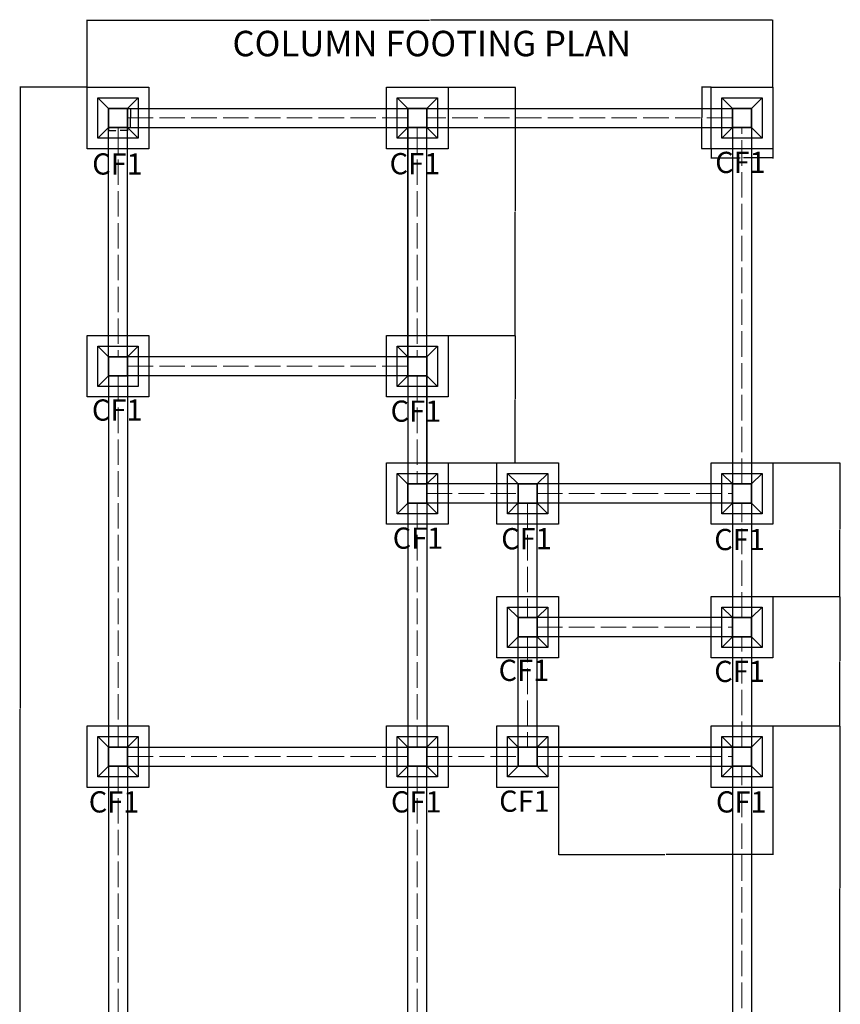
# Model space of a CAD drawing. Units: inches. Extents: x -154 to 668, y -797 to 97.
# Tile 4 of 4: x 282 to 668, y -367 to 97. Entities that reach past the tile are written whole.
import ezdxf

# ---------------------------------------------------------------- set-up
doc = ezdxf.new("R2010")
doc.units = ezdxf.units.IN
doc.header["$MEASUREMENT"] = 0
doc.linetypes.add('ACAD_ISO02W100', pattern=[15, 12, -3])
for name, color, linetype, lineweight in [('A-ANNO-DIMS', 2, 'Continuous', 18), ('A-ANNO-TITL', 1, 'Continuous', 30), ('S-ANNO-IDEN', 7, 'Continuous', 18), ('S-BEAM', 152, 'Continuous', 25), ('S-BEAM-CNTR', 2, 'ACAD_ISO02W100', 13), ('S-COLS', 2, 'Continuous', 35), ('S-FNDN', 2, 'Continuous', 30)]:
    doc.layers.add(name, color=color, linetype=linetype, lineweight=lineweight)
doc.styles.get("Standard").update_dxf_attribs({"font": 'arial.ttf'})
doc.dimstyles.get("Standard").update_dxf_attribs({"dimtxt": 0.18, "dimasz": 0.18, "dimexe": 0.18, "dimexo": 0.0625, "dimgap": 0.09, "dimtad": 0, "dimtih": 1, "dimtoh": 1, "dimdec": 1, "dimzin": 0, "dimdsep": 46, "dimlunit": 4, "dimtxsty": 'Standard', "dimcen": 0.09, "dimadec": 0, "dimazin": 0, "dimtfac": 1, "dimtdec": 1, "dimtofl": 0, "dimtmove": 0, "dimatfit": 3, "dimfxl": 1, "dimtolj": 1, "dimtzin": 0, "dimarcsym": 0})

# ---------------------------------------------------------------- blocks, each defined once
blk = doc.blocks.new('COLUMN-9X9')
for p, q in [((-4.5, 4.5), (4.5, 4.5)), ((-4.5, -4.5), (-4.5, 4.5)), ((4.5, 4.5), (4.5, -4.5)), ((4.5, -4.5), (-4.5, -4.5))]:
    blk.add_line(p, q)
blk = doc.blocks.new('CF1-ISOLATED-FOOTING')
for p, q in [((-14.5, 14.5), (14.5, 14.5)), ((-14.5, -14.5), (-14.5, 14.5)), ((14.5, 14.5), (14.5, -14.5)), ((-9.5, 9.5), (9.5, 9.5)), ((-9.5, -9.5), (-9.5, 9.5)), ((-9.5, 9.5), (-4.5, 4.5)), ((4.5, 4.5), (9.5, 9.5)), ((9.5, 9.5), (9.5, -9.5)), ((-9.5, -9.5), (-4.5, -4.5)), ((4.5, -4.5), (9.5, -9.5)), ((9.5, -9.5), (-9.5, -9.5)), ((14.5, -14.5), (-14.5, -14.5))]:
    blk.add_line(p, q)
blk = doc.blocks.new('*D23')
at = {"layer": 'A-ANNO-DIMS', "color": 0, "lineweight": -2, "transparency": 16777216}
for p, q in [((323.4, 46.27), (323.4, 44.8)), ((323.58, 44.98), (326.86, 44.98)), ((332.22, 44.98), (328.94, 44.98)), ((332.4, 46.27), (332.4, 44.8))]:
    blk.add_line(p, q, dxfattribs=at)
at = {"layer": 'A-ANNO-DIMS', "color": 0, "transparency": 16777216}
for points in [[(323.58, 45.01), (323.58, 44.95), (323.4, 44.98)], [(332.22, 45.01), (332.22, 44.95), (332.4, 44.98)]]:
    blk.add_solid(points, dxfattribs=at)
at = {"layer": 'Defpoints', "color": 0, "transparency": 16777216}
for p in [(323.4, 46.33), (332.4, 46.33), (332.4, 44.98)]:
    blk.add_point(p, dxfattribs=at)
at = {"layer": 'A-ANNO-DIMS', "color": 0, "transparency": 16777216, "insert": (327.9, 44.98), "char_height": 0.18, "attachment_point": 5}
blk.add_mtext('\\A1;COLUMN 9 TYP.', dxfattribs=at)
blk = doc.blocks.new('*D24')
at = {"layer": 'A-ANNO-DIMS', "color": 0, "lineweight": -2, "transparency": 16777216}
for p, q in [((332.46, 55.33), (333.93, 55.33)), ((333.75, 55.15), (333.75, 51.01)), ((333.75, 46.51), (333.75, 50.65)), ((332.46, 46.33), (333.93, 46.33))]:
    blk.add_line(p, q, dxfattribs=at)
at = {"layer": 'A-ANNO-DIMS', "color": 0, "transparency": 16777216}
for points in [[(333.72, 55.15), (333.78, 55.15), (333.75, 55.33)], [(333.72, 46.51), (333.78, 46.51), (333.75, 46.33)]]:
    blk.add_solid(points, dxfattribs=at)
at = {"layer": 'Defpoints', "color": 0, "transparency": 16777216}
for p in [(332.4, 55.33), (333.75, 55.33), (332.4, 46.33)]:
    blk.add_point(p, dxfattribs=at)
at = {"layer": 'A-ANNO-DIMS', "color": 0, "transparency": 16777216, "insert": (333.75, 50.83), "char_height": 0.18, "attachment_point": 5}
blk.add_mtext('\\A1;9 TYP.', dxfattribs=at)
blk = doc.blocks.new('*D25')
at = {"layer": 'A-ANNO-DIMS', "color": 0, "lineweight": -2, "transparency": 16777216}
for p, q in [((607.4, 36.27), (607.4, 31.8)), ((636.4, 36.27), (636.4, 31.8)), ((607.58, 31.98), (621.1, 31.98)), ((636.22, 31.98), (622.7, 31.98))]:
    blk.add_line(p, q, dxfattribs=at)
at = {"layer": 'A-ANNO-DIMS', "color": 0, "transparency": 16777216}
for points in [[(607.58, 32.01), (607.58, 31.95), (607.4, 31.98)], [(636.22, 32.01), (636.22, 31.95), (636.4, 31.98)]]:
    blk.add_solid(points, dxfattribs=at)
at = {"layer": 'Defpoints', "color": 0, "transparency": 16777216}
for p in [(607.4, 36.33), (636.4, 36.33), (636.4, 31.98)]:
    blk.add_point(p, dxfattribs=at)
at = {"layer": 'A-ANNO-DIMS', "color": 0, "transparency": 16777216, "insert": (621.9, 31.98), "char_height": 0.18, "attachment_point": 5}
blk.add_mtext('\\A1;CF1 29 TYP.', dxfattribs=at)
blk = doc.blocks.new('*D26')
at = {"layer": 'A-ANNO-DIMS', "color": 0, "lineweight": -2, "transparency": 16777216}
for p, q in [((607.34, 65.33), (602.87, 65.33)), ((603.05, 65.15), (603.05, 51.01)), ((603.05, 36.51), (603.05, 50.65)), ((607.34, 36.33), (602.87, 36.33))]:
    blk.add_line(p, q, dxfattribs=at)
at = {"layer": 'A-ANNO-DIMS', "color": 0, "transparency": 16777216}
for points in [[(603.02, 65.15), (603.08, 65.15), (603.05, 65.33)], [(603.02, 36.51), (603.08, 36.51), (603.05, 36.33)]]:
    blk.add_solid(points, dxfattribs=at)
at = {"layer": 'Defpoints', "color": 0, "transparency": 16777216}
for p in [(607.4, 65.33), (603.05, 36.33), (607.4, 36.33)]:
    blk.add_point(p, dxfattribs=at)
at = {"layer": 'A-ANNO-DIMS', "color": 0, "transparency": 16777216, "insert": (603.05, 50.83), "char_height": 0.18, "attachment_point": 5}
blk.add_mtext('\\A1;29 TYP.', dxfattribs=at)
blk = doc.blocks.new('*D50')
at = {"layer": 'A-ANNO-DIMS', "color": 0, "lineweight": -2, "transparency": 16777216}
for p, q in [((313.4, 65.4), (313.4, 97.16)), ((313.58, 96.98), (474.61, 96.98)), ((636.22, 96.98), (475.19, 96.98)), ((636.4, 65.4), (636.4, 97.16))]:
    blk.add_line(p, q, dxfattribs=at)
at = {"layer": 'A-ANNO-DIMS', "color": 0, "transparency": 16777216}
for points in [[(313.58, 97.01), (313.58, 96.95), (313.4, 96.98)], [(636.22, 97.01), (636.22, 96.95), (636.4, 96.98)]]:
    blk.add_solid(points, dxfattribs=at)
at = {"layer": 'Defpoints', "color": 0, "transparency": 16777216}
for p in [(636.4, 96.98), (313.4, 65.33), (636.4, 65.33)]:
    blk.add_point(p, dxfattribs=at)
at = {"layer": 'A-ANNO-DIMS', "color": 0, "transparency": 16777216, "insert": (474.9, 96.98), "char_height": 0.18, "attachment_point": 5}
blk.add_mtext('\\A1;323', dxfattribs=at)
blk = doc.blocks.new('*D51')
at = {"layer": 'A-ANNO-DIMS', "color": 0, "lineweight": -2, "transparency": 16777216}
for p, q in [((313.34, 65.33), (281.57, 65.33)), ((281.75, 65.15), (281.75, -227.49)), ((281.75, -520.49), (281.75, -227.85)), ((313.34, -520.67), (281.57, -520.67))]:
    blk.add_line(p, q, dxfattribs=at)
at = {"layer": 'A-ANNO-DIMS', "color": 0, "transparency": 16777216}
for points in [[(281.72, 65.15), (281.78, 65.15), (281.75, 65.33)], [(281.72, -520.49), (281.78, -520.49), (281.75, -520.67)]]:
    blk.add_solid(points, dxfattribs=at)
at = {"layer": 'Defpoints', "color": 0, "transparency": 16777216}
for p in [(281.75, 65.33), (313.4, 65.33), (313.4, -520.67)]:
    blk.add_point(p, dxfattribs=at)
at = {"layer": 'A-ANNO-DIMS', "color": 0, "transparency": 16777216, "insert": (281.75, -227.67), "char_height": 0.18, "attachment_point": 5}
blk.add_mtext('\\A1;586', dxfattribs=at)
blk = doc.blocks.new('*D54')
at = {"layer": 'A-ANNO-DIMS', "color": 0, "lineweight": -2, "transparency": 16777216}
for p, q in [((535.4, -264.73), (535.4, -296.5)), ((636.4, -264.73), (636.4, -296.5)), ((535.58, -296.32), (585.64, -296.32)), ((636.22, -296.32), (586.16, -296.32))]:
    blk.add_line(p, q, dxfattribs=at)
at = {"layer": 'A-ANNO-DIMS', "color": 0, "transparency": 16777216}
for points in [[(535.58, -296.29), (535.58, -296.35), (535.4, -296.32)], [(636.22, -296.29), (636.22, -296.35), (636.4, -296.32)]]:
    blk.add_solid(points, dxfattribs=at)
at = {"layer": 'Defpoints', "color": 0, "transparency": 16777216}
for p in [(535.4, -264.67), (636.4, -264.67), (535.4, -296.32)]:
    blk.add_point(p, dxfattribs=at)
at = {"layer": 'A-ANNO-DIMS', "color": 0, "transparency": 16777216, "insert": (585.9, -296.32), "char_height": 0.18, "attachment_point": 5}
blk.add_mtext('\\A1;101', dxfattribs=at)
blk = doc.blocks.new('*D55')
at = {"layer": 'A-ANNO-DIMS', "color": 0, "lineweight": -2, "transparency": 16777216}
for p, q in [((483.46, 65.33), (515.23, 65.33)), ((515.05, 65.15), (515.05, 7.01)), ((515.05, -51.49), (515.05, 6.65)), ((483.46, -51.67), (515.23, -51.67))]:
    blk.add_line(p, q, dxfattribs=at)
at = {"layer": 'A-ANNO-DIMS', "color": 0, "transparency": 16777216}
for points in [[(515.02, 65.15), (515.08, 65.15), (515.05, 65.33)], [(515.02, -51.49), (515.08, -51.49), (515.05, -51.67)]]:
    blk.add_solid(points, dxfattribs=at)
at = {"layer": 'Defpoints', "color": 0, "transparency": 16777216}
for p in [(483.4, 65.33), (483.4, -51.67), (515.05, -51.67)]:
    blk.add_point(p, dxfattribs=at)
at = {"layer": 'A-ANNO-DIMS', "color": 0, "transparency": 16777216, "insert": (515.05, 6.83), "char_height": 0.18, "attachment_point": 5}
blk.add_mtext('\\A1;117', dxfattribs=at)
blk = doc.blocks.new('*D56')
at = {"layer": 'A-ANNO-DIMS', "color": 0, "lineweight": -2, "transparency": 16777216}
for p, q in [((483.46, -51.67), (515.23, -51.67)), ((515.05, -51.85), (515.05, -81.49)), ((515.05, -111.49), (515.05, -81.85)), ((483.46, -111.67), (515.23, -111.67))]:
    blk.add_line(p, q, dxfattribs=at)
at = {"layer": 'A-ANNO-DIMS', "color": 0, "transparency": 16777216}
for points in [[(515.02, -51.85), (515.08, -51.85), (515.05, -51.67)], [(515.02, -111.49), (515.08, -111.49), (515.05, -111.67)]]:
    blk.add_solid(points, dxfattribs=at)
at = {"layer": 'Defpoints', "color": 0, "transparency": 16777216}
for p in [(483.4, -51.67), (483.4, -111.67), (515.05, -111.67)]:
    blk.add_point(p, dxfattribs=at)
at = {"layer": 'A-ANNO-DIMS', "color": 0, "transparency": 16777216, "insert": (515.05, -81.67), "char_height": 0.18, "attachment_point": 5}
blk.add_mtext('\\A1;60', dxfattribs=at)
blk = doc.blocks.new('*D57')
at = {"layer": 'A-ANNO-DIMS', "color": 0, "lineweight": -2, "transparency": 16777216}
for p, q in [((636.46, -111.67), (668.23, -111.67)), ((668.05, -111.85), (668.05, -142.99)), ((668.05, -174.49), (668.05, -143.35)), ((636.46, -174.67), (668.23, -174.67))]:
    blk.add_line(p, q, dxfattribs=at)
at = {"layer": 'A-ANNO-DIMS', "color": 0, "transparency": 16777216}
for points in [[(668.02, -111.85), (668.08, -111.85), (668.05, -111.67)], [(668.02, -174.49), (668.08, -174.49), (668.05, -174.67)]]:
    blk.add_solid(points, dxfattribs=at)
at = {"layer": 'Defpoints', "color": 0, "transparency": 16777216}
for p in [(636.4, -111.67), (668.05, -111.67), (636.4, -174.67)]:
    blk.add_point(p, dxfattribs=at)
at = {"layer": 'A-ANNO-DIMS', "color": 0, "transparency": 16777216, "insert": (668.05, -143.17), "char_height": 0.18, "attachment_point": 5}
blk.add_mtext('\\A1;63', dxfattribs=at)
blk = doc.blocks.new('*D58')
at = {"layer": 'A-ANNO-DIMS', "color": 0, "lineweight": -2, "transparency": 16777216}
for p, q in [((636.46, -174.67), (668.23, -174.67)), ((668.05, -174.85), (668.05, -204.99)), ((668.05, -235.49), (668.05, -205.35)), ((636.46, -235.67), (668.23, -235.67))]:
    blk.add_line(p, q, dxfattribs=at)
at = {"layer": 'A-ANNO-DIMS', "color": 0, "transparency": 16777216}
for points in [[(668.02, -174.85), (668.08, -174.85), (668.05, -174.67)], [(668.02, -235.49), (668.08, -235.49), (668.05, -235.67)]]:
    blk.add_solid(points, dxfattribs=at)
at = {"layer": 'Defpoints', "color": 0, "transparency": 16777216}
for p in [(636.4, -174.67), (668.05, -174.67), (636.4, -235.67)]:
    blk.add_point(p, dxfattribs=at)
at = {"layer": 'A-ANNO-DIMS', "color": 0, "transparency": 16777216, "insert": (668.05, -205.17), "char_height": 0.18, "attachment_point": 5}
blk.add_mtext('\\A1;61', dxfattribs=at)
blk = doc.blocks.new('*D59')
at = {"layer": 'A-ANNO-DIMS', "color": 0, "lineweight": -2, "transparency": 16777216}
for p, q in [((636.46, -235.67), (668.23, -235.67)), ((668.05, -235.85), (668.05, -311.99)), ((668.05, -388.49), (668.05, -312.35)), ((636.46, -388.67), (668.23, -388.67))]:
    blk.add_line(p, q, dxfattribs=at)
at = {"layer": 'A-ANNO-DIMS', "color": 0, "transparency": 16777216}
for points in [[(668.02, -235.85), (668.08, -235.85), (668.05, -235.67)], [(668.02, -388.49), (668.08, -388.49), (668.05, -388.67)]]:
    blk.add_solid(points, dxfattribs=at)
at = {"layer": 'Defpoints', "color": 0, "transparency": 16777216}
for p in [(636.4, -235.67), (668.05, -235.67), (636.4, -388.67)]:
    blk.add_point(p, dxfattribs=at)
at = {"layer": 'A-ANNO-DIMS', "color": 0, "transparency": 16777216, "insert": (668.05, -312.17), "char_height": 0.18, "attachment_point": 5}
blk.add_mtext('\\A1;153', dxfattribs=at)

msp = doc.modelspace()

# ---------------------------------------------------------------- linework, layer by layer
at = {"layer": 'S-BEAM'}
for p, q in [((323.3997, 55.3328), (473.3997, 55.3328)), ((323.3997, -70.6672), (323.3997, 55.3328)), ((473.3997, 55.3328), (626.3997, 55.3328)), ((626.3997, 55.3328), (626.3997, -130.6672)), ((332.3997, 46.3328), (464.3997, 46.3328)), ((332.3997, -61.6672), (332.3997, 46.3328)), ((464.3997, 46.3328), (464.3997, -61.6672)), ((464.3997, -61.6672), (464.3997, 46.3328)), ((473.3997, 46.3328), (617.3997, 46.3328)), ((473.3997, -121.6672), (473.3997, 46.3328)), ((617.3997, 46.3328), (617.3997, -121.6672)), ((464.3997, -61.6672), (332.3997, -61.6672)), ((323.3997, -70.6672), (323.3997, -254.6672)), ((464.3997, -70.6672), (332.3997, -70.6672)), ((332.3997, -70.6672), (332.3997, -245.6672)), ((464.3997, -70.6672), (464.3997, -245.6672)), ((473.3997, -70.6672), (473.3997, -121.6672)), ((473.3997, -70.6672), (473.3997, -245.6672)), ((617.3997, -121.6672), (473.3997, -121.6672)), ((516.3997, -130.6672), (464.3997, -130.6672)), ((516.3997, -184.6672), (516.3997, -130.6672)), ((617.3997, -130.6672), (525.3997, -130.6672)), ((525.3997, -184.6672), (525.3997, -130.6672)), ((617.3997, -130.6672), (617.3997, -184.6672)), ((626.3997, -130.6672), (626.3997, -193.6672)), ((516.3997, -245.6672), (516.3997, -184.6672)), ((617.3997, -184.6672), (525.3997, -184.6672)), ((617.3997, -193.6672), (525.3997, -193.6672)), ((525.3997, -245.6672), (525.3997, -193.6672)), ((617.3997, -193.6672), (617.3997, -245.6672)), ((626.3997, -193.6672), (626.3997, -254.6672)), ((332.3997, -245.6672), (473.3997, -245.6672)), ((473.3997, -245.6672), (516.3997, -245.6672)), ((617.3997, -245.6672), (525.3997, -245.6672)), ((525.3997, -245.6672), (617.3997, -245.6672)), ((323.3997, -254.6672), (323.3997, -407.6672)), ((332.3997, -254.6672), (617.3997, -254.6672)), ((332.3997, -254.6672), (332.3997, -398.6672)), ((464.3997, -398.6672), (464.3997, -254.6672)), ((473.3997, -398.6672), (473.3997, -254.6672)), ((473.3997, -254.6672), (617.3997, -254.6672)), ((617.3997, -254.6672), (617.3997, -398.6672)), ((626.3997, -254.6672), (626.3997, -510.6672))]:
    msp.add_line(p, q, dxfattribs=at)
at = {"layer": 'S-BEAM-CNTR'}
for p, q in [((464.3997, 50.8328), (332.3997, 50.8328)), ((617.3997, 50.8328), (473.3997, 50.8328)), ((327.8997, 46.3328), (327.8997, -61.6672)), ((468.8997, 46.3328), (468.8997, -61.6672)), ((621.8997, -121.6672), (621.8997, 46.3328)), ((332.3997, -66.1672), (464.3997, -66.1672)), ((327.8997, -70.6672), (327.8997, -245.6672)), ((468.8997, -70.6672), (468.8997, -121.6672)), ((473.3997, -126.1672), (516.3997, -126.1672)), ((525.3997, -126.1672), (617.3997, -126.1672)), ((468.8997, -130.6672), (468.8997, -245.6672)), ((520.8997, -130.6672), (520.8997, -184.6672)), ((621.8997, -184.6672), (621.8997, -130.6672)), ((525.3997, -189.1672), (617.3997, -189.1672)), ((520.8997, -193.6672), (520.8997, -245.6672)), ((621.8997, -245.6672), (621.8997, -193.6672)), ((332.3997, -250.1672), (464.3997, -250.1672)), ((473.3997, -250.1672), (516.3997, -250.1672)), ((525.3997, -250.1672), (617.3997, -250.1672)), ((327.8997, -254.6672), (327.8997, -398.6672)), ((468.8997, -254.6672), (468.8997, -398.6672)), ((621.8997, -398.6672), (621.8997, -254.6672))]:
    msp.add_line(p, q, dxfattribs=at)
at = {"layer": 'S-COLS'}
msp.add_line((525.3997, -184.6672), (525.3997, -193.6672), dxfattribs=at)
at = {"layer": 'S-FNDN'}
for p, q in [((313.3997, -51.6672), (342.3997, -51.6672)), ((313.3997, -80.6672), (313.3997, -51.6672)), ((342.3997, -51.6672), (342.3997, -80.6672)), ((318.3997, -56.6672), (337.3997, -56.6672)), ((318.3997, -75.6672), (318.3997, -56.6672)), ((318.3997, -56.6672), (323.3997, -61.6672)), ((332.3997, -61.6672), (337.3997, -56.6672)), ((337.3997, -56.6672), (337.3997, -75.6672)), ((318.3997, -75.6672), (323.3997, -70.6672)), ((337.3997, -75.6672), (318.3997, -75.6672)), ((342.3997, -80.6672), (313.3997, -80.6672)), ((454.3997, -140.6672), (454.3997, -111.6672)), ((454.3997, -111.6672), (483.3997, -111.6672)), ((483.3997, -111.6672), (483.3997, -140.6672)), ((506.3997, -140.6672), (506.3997, -111.6672)), ((506.3997, -111.6672), (535.3997, -111.6672)), ((535.3997, -111.6672), (535.3997, -140.6672)), ((459.3997, -135.6672), (459.3997, -116.6672)), ((459.3997, -116.6672), (478.3997, -116.6672)), ((459.3997, -116.6672), (464.635, -121.8886)), ((473.3997, -121.6672), (478.3997, -116.6672)), ((478.3997, -116.6672), (478.3997, -135.6672)), ((511.3997, -135.6672), (511.3997, -116.6672)), ((511.3997, -116.6672), (530.3997, -116.6672)), ((511.3997, -116.6672), (516.3997, -121.6672)), ((525.3997, -121.6672), (530.3997, -116.6672)), ((530.3997, -116.6672), (530.3997, -135.6672)), ((459.3997, -135.6672), (464.3997, -130.6672)), ((473.3997, -130.6672), (478.3997, -135.6672)), ((511.3997, -135.6672), (516.5981, -130.4343)), ((525.3997, -130.6672), (530.3997, -135.6672)), ((478.3997, -135.6672), (459.3997, -135.6672)), ((530.3997, -135.6672), (511.3997, -135.6672)), ((483.3997, -140.6672), (454.3997, -140.6672)), ((535.3997, -140.6672), (506.3997, -140.6672))]:
    msp.add_line(p, q, dxfattribs=at)

# ---------------------------------------------------------------- block references
at = {"layer": 'S-COLS'}
msp.add_blockref('COLUMN-9X9', (327.9, 50.833), dxfattribs=at)
for p, rotation in [((468.8995, 50.8331), 90.00000000000036), ((621.8995, 50.8331), 90), ((327.8995, -66.1669), 89.99999999999928), ((468.8995, -66.1669), 90.00000000000036), ((468.8995, -126.1669), 90.00000000000055), ((520.8995, -126.1669), 90.00000000000018), ((621.8995, -126.1669), 90.00000000000018), ((520.8995, -189.1669), 90), ((621.8995, -189.1669), 90), ((327.8995, -250.1669), 89.9999999999991), ((468.8995, -250.1669), 90.00000000000036), ((520.8995, -250.1669), 90), ((621.8995, -250.1669), 90)]:
    msp.add_blockref('COLUMN-9X9', p, dxfattribs=dict(at, rotation=rotation))
at = {"layer": 'S-FNDN'}
for p in [(327.9, 50.833), (520.9, -189.167), (327.9, -250.167)]:
    msp.add_blockref('CF1-ISOLATED-FOOTING', p, dxfattribs=at)
for p, rotation in [((468.8995, 50.8331), 90), ((621.8999, 50.8325), 269.9999999999997), ((468.8994, -66.1674), 180), ((621.8994, -126.1674), 180), ((621.8994, -189.1674), 180), ((468.8995, -250.1669), 90), ((520.8995, -250.1669), 90), ((621.8994, -250.1674), 180)]:
    msp.add_blockref('CF1-ISOLATED-FOOTING', p, dxfattribs=dict(at, rotation=rotation))

# ---------------------------------------------------------------- texts
at = {"layer": 'A-ANNO-TITL'}
msp.add_text('COLUMN FOOTING PLAN', height=12, dxfattribs=at).set_placement((381.8106, 79.9286))
at = {"layer": 'S-ANNO-IDEN'}
for p in [(315.6995, 24.1633), (455.8568, 24.2968), (609.2884, 24.8957), (315.5683, -91.8086), (456.3283, -92.3322), (457.3214, -152.1864), (508.4542, -152.467), (608.8568, -152.845), (507.2405, -214.4893), (608.8568, -214.9927), (314.0868, -276.5002), (456.5079, -276.4891), (507.4953, -276.1501), (609.63, -276.5053)]:
    msp.add_text('CF1', height=10, dxfattribs=at).set_placement(p)

# ---------------------------------------------------------------- dimensions: what is measured, and where the dimension line sits
at = {"layer": 'A-ANNO-DIMS'}
dim = msp.add_linear_dim(base=(636.3997, 96.9828), p1=(313.3997, 65.3328), p2=(636.3997, 65.3328), dimstyle='Standard', override={"dimdec": 0, "dimlfac": 1, "dimrnd": 0, "dimzin": 0, "dimdsep": 46, "dimlunit": 2}, dxfattribs=at)
dim.commit()
dim.dimension.update_dxf_attribs({"geometry": '*D50', "text_midpoint": (474.8997, 96.9828)})
for base, p1, p2, angle, picture, middle in [((281.7497, 65.3328), (313.3997, -520.6672), (313.3997, 65.3328), 90, '*D51', (281.7497, -227.6672)), ((515.0497, -51.6672), (483.3997, 65.3328), (483.3997, -51.6672), 270, '*D55', (515.0497, 6.8328)), ((515.0497, -111.6672), (483.3997, -51.6672), (483.3997, -111.6672), 270, '*D56', (515.0497, -81.6672)), ((668.0497, -111.6672), (636.3997, -174.6672), (636.3997, -111.6672), 90, '*D57', (668.0497, -143.1672)), ((668.0497, -174.6672), (636.3997, -235.6672), (636.3997, -174.6672), 90, '*D58', (668.0497, -205.1672)), ((668.0497, -235.6672), (636.3997, -388.6672), (636.3997, -235.6672), 90, '*D59', (668.0497, -312.1672)), ((535.3997, -296.3172), (636.3997, -264.6672), (535.3997, -264.6672), 180, '*D54', (585.8997, -296.3172))]:
    dim = msp.add_linear_dim(base=base, p1=p1, p2=p2, angle=angle, dimstyle='Standard', override={"dimdec": 0, "dimlfac": 1, "dimrnd": 0, "dimzin": 0, "dimdsep": 46, "dimlunit": 2}, dxfattribs=at)
    dim.commit()
    dim.dimension.update_dxf_attribs({"geometry": picture, "text_midpoint": middle})
for base, p1, p2, angle, picture, middle in [((603.0497, 36.3328), (607.3997, 65.3328), (607.3997, 36.3328), 270, '*D26', (603.0497, 50.8328)), ((333.7497, 55.3328), (332.3997, 46.3328), (332.3997, 55.3328), 90, '*D24', (333.7497, 50.8328))]:
    dim = msp.add_linear_dim(base=base, p1=p1, p2=p2, angle=angle, text='<> TYP.', dimstyle='Standard', override={"dimdec": 0, "dimlfac": 1, "dimrnd": 0, "dimzin": 0, "dimdsep": 46, "dimlunit": 2}, dxfattribs=at)
    dim.commit()
    dim.dimension.update_dxf_attribs({"geometry": picture, "text_midpoint": middle})
for base, p1, p2, text, picture, middle in [((332.3997, 44.9828), (323.3997, 46.3328), (332.3997, 46.3328), 'COLUMN <> TYP.', '*D23', (327.8997, 44.9828)), ((636.3997, 31.9828), (607.3997, 36.3328), (636.3997, 36.3328), 'CF1 <> TYP.', '*D25', (621.8997, 31.9828))]:
    dim = msp.add_linear_dim(base=base, p1=p1, p2=p2, text=text, dimstyle='Standard', override={"dimdec": 0, "dimlfac": 1, "dimrnd": 0, "dimzin": 0, "dimdsep": 46, "dimlunit": 2}, dxfattribs=at)
    dim.commit()
    dim.dimension.update_dxf_attribs({"geometry": picture, "text_midpoint": middle})

doc.saveas('drawing.dxf')
